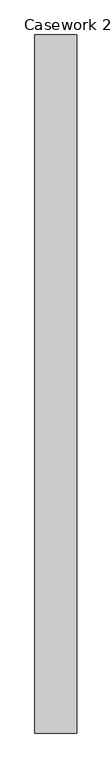
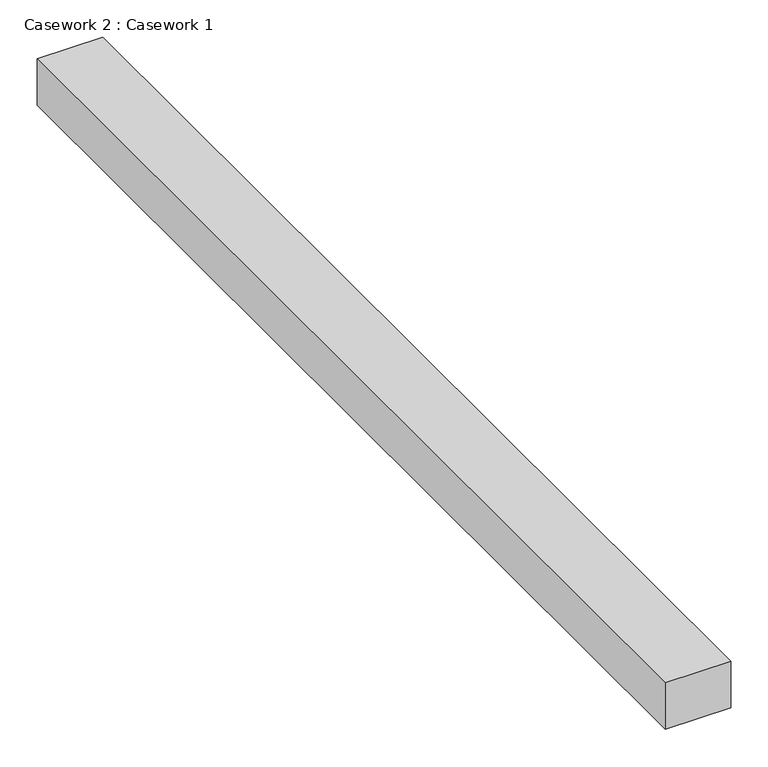
"""IFC4 building model written with IfcOpenShell, lengths in millimetres: furniture geometry, Casework 2 : Casework 1."""

from ifc_helpers import new_model, si_unit, frame, origin, place, context, project, spatial, polyline, outline, extrude, source, transform, mapped, element, save


def casework_2_casework_1_1fe19027(model_context):
    return source(origin(), model_context, "Body", "SweptSolid", [
        extrude(outline(polyline([(9357.7559589, 14787.9496924), (9357.7559589, 13098.8496924), (9256.1559589, 13098.8496924), (9256.1559589, 14787.9496924), (9357.7559589, 14787.9496924)])), frame((0.0, 0.0, 3581.4), z_axis=(0.0, 0.0, 1.0), x_axis=(1.0, 0.0, 0.0)), (0.0, 0.0, 1.0), 76.2),
    ])


if __name__ == "__main__":
    model = new_model("IFC4")
    model_context = context("Model", 3, world=origin())
    ifc_project = project(units=[si_unit("LENGTHUNIT", "METRE", prefix="MILLI")], contexts=[model_context])
    site = spatial("IfcSite", under=ifc_project)
    building = spatial("IfcBuilding", under=site)
    placement = place(None, origin())
    casework_2_casework_1_shape = casework_2_casework_1_1fe19027(model_context)
    element("IfcFurniture", 1, ObjectType="Casework 2 : Casework 1", at=placement, inside=building, context=model_context, shape_type="MappedRepresentation", body=[
        mapped(casework_2_casework_1_shape, transform((0.0, 0.0, 0.0), x_axis=(1.0, 0.0, 0.0), y_axis=(0.0, 1.0, 0.0), z_axis=(0.0, 0.0, 1.0))),
    ])
    save(model, "model.ifc")

# Revit data of these elements
# Element 1 (IfcFurniture, "Casework 2 : Casework 1")
#   Materials on its faces: "Clad - White"
# Materials
#   "Clad - White": class "Wood", colour RGB 242 242 238, transparency 0, Cost = 0
